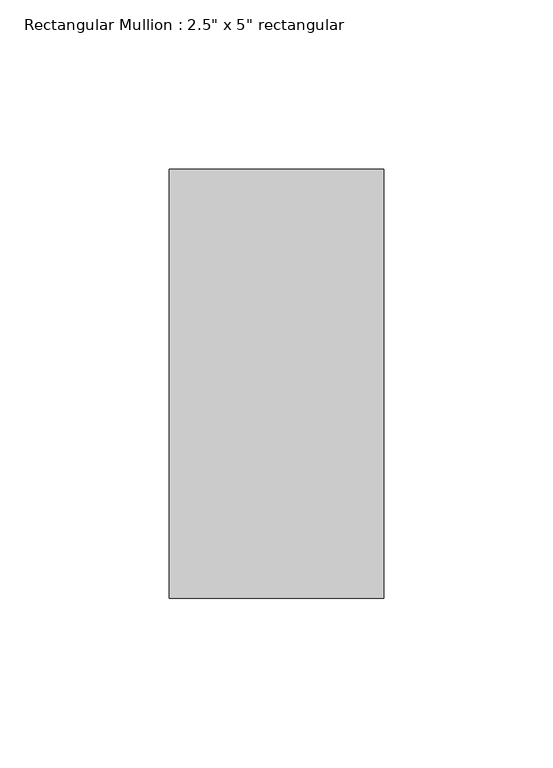
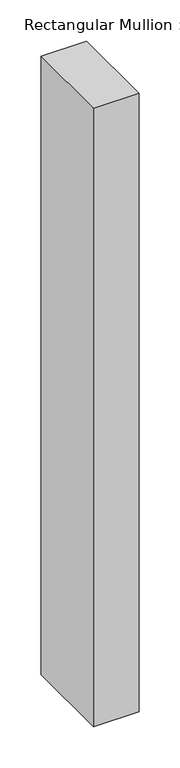
"""IFC4 building model written with IfcOpenShell, lengths in millimetres: member geometry."""

from ifc_helpers import new_model, si_unit, frame, origin, place, context, project, spatial, polyline, outline, extrude, source, transform, mapped, element, save


def member_73c23c35(model_context):
    return source(origin(), model_context, "Body", "SweptSolid", [
        extrude(outline(polyline([(0.0, 63.5), (0.0, -63.5), (-63.5, -63.5), (-63.5, 63.5), (0.0, 63.5)])), frame((0.0, 0.0, -914.4), z_axis=(0.0, 0.0, 1.0), x_axis=(1.0, 0.0, 0.0)), (0.0, 0.0, 1.0), 914.4),
    ])


if __name__ == "__main__":
    model = new_model("IFC4")
    model_context = context("Model", 3, world=origin())
    ifc_project = project(units=[si_unit("LENGTHUNIT", "METRE", prefix="MILLI")], contexts=[model_context])
    site = spatial("IfcSite", under=ifc_project)
    building = spatial("IfcBuilding", under=site)
    placement = place(None, origin())
    member_shape = member_73c23c35(model_context)
    element("IfcMember", 1, ObjectType="Rectangular Mullion : 2.5\" x 5\" rectangular", at=placement, inside=building, context=model_context, shape_type="MappedRepresentation", body=[
        mapped(member_shape, transform((0.0, 0.0, 0.0), x_axis=(1.0, 0.0, 0.0), y_axis=(0.0, 1.0, 0.0), z_axis=(0.0, 0.0, 1.0))),
    ])
    save(model, "model.ifc")

# Revit data of these elements
# Type "Rectangular Mullion : 2.5\" x 5\" rectangular"
#   built-in parameter 1007304 = 0.416667 (stored number, unit not read)
#   built-in parameter 1007301 = 0.104167 (stored number, unit not read)
#   built-in parameter 1007300 = 0.104167 (stored number, unit not read)
# Element 1 (IfcMember, "Rectangular Mullion : 2.5\" x 5\" rectangular")
#   Materials on its faces: "Iron, Ductile"
# Materials
#   "Iron, Ductile": class "Metal", colour RGB 0 0 0, transparency 0, Description = "Ductile cast iron", Cost = 0
